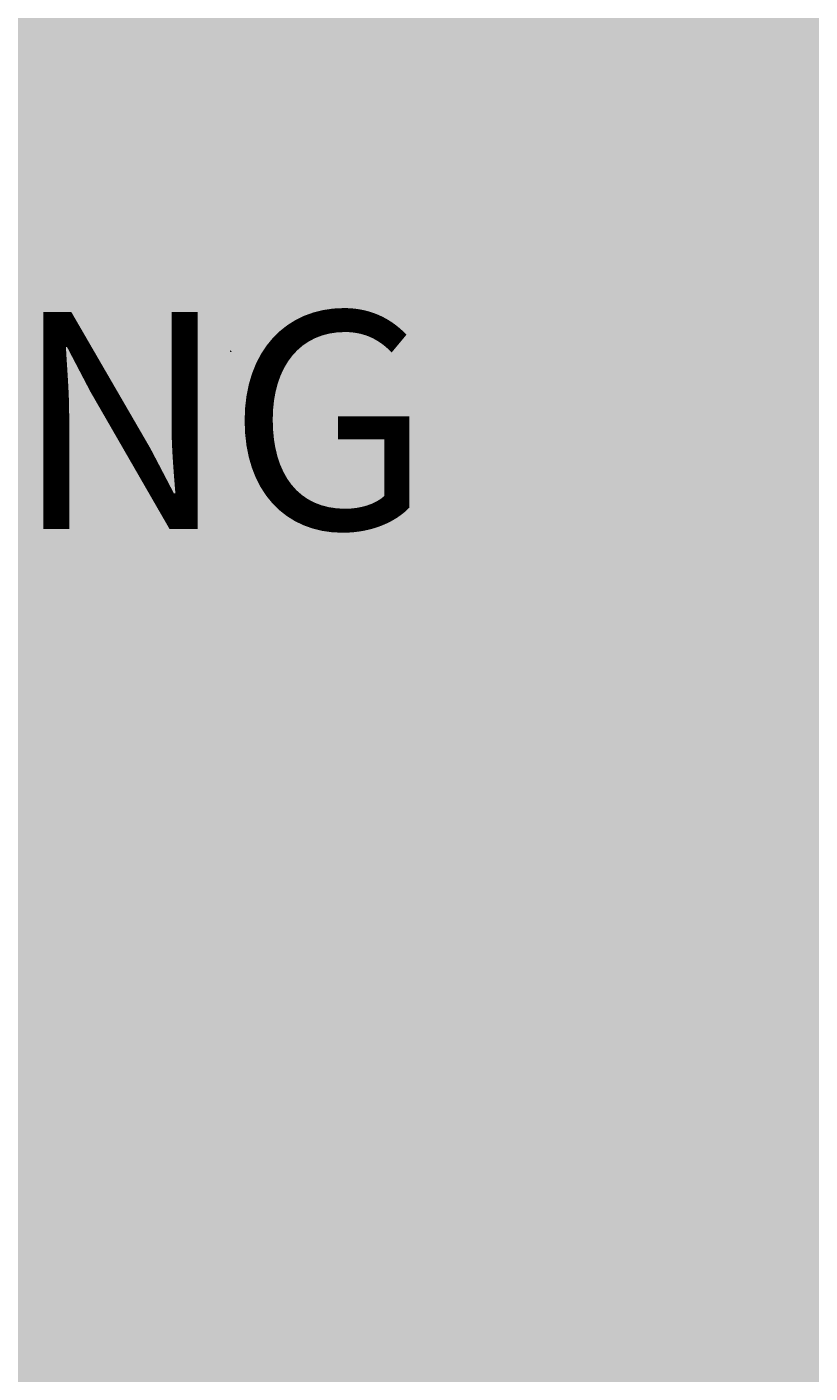
# Model space of a CAD drawing. Units: millimetres. Extents: x -229 to 16545, y -10488 to 4272.
# Tile 14 of 29: x 10978 to 11804, y -4126 to -2708. Entities that reach past the tile are written whole.
import ezdxf

# ---------------------------------------------------------------- set-up
doc = ezdxf.new("R2010")
doc.units = ezdxf.units.MM
doc.layers.add('A-ANNO-DIMS', color=2, linetype='Continuous', lineweight=18)
doc.layers.add('A-AREA-IDEN', color=7, linetype='Continuous', lineweight=18)
doc.layers.add('A-FLOR-PATT', color=254, linetype='Continuous', lineweight=13, true_color=0xfeeab9)
doc.styles.get("Standard").update_dxf_attribs({"font": 'arial.ttf'})
doc.dimstyles.get("Standard").update_dxf_attribs({"dimtxt": 0.18, "dimasz": 0.18, "dimexe": 0.18, "dimexo": 0.0625, "dimgap": 0.09, "dimtad": 0, "dimtih": 1, "dimtoh": 1, "dimdec": 4, "dimzin": 0, "dimdsep": 46, "dimtxsty": 'Standard', "dimcen": 0.09, "dimadec": 0, "dimazin": 0, "dimtfac": 1, "dimtdec": 4, "dimtofl": 0, "dimtmove": 0, "dimatfit": 3, "dimfxl": 1, "dimtolj": 1, "dimtzin": 0, "dimarcsym": 0})

# ---------------------------------------------------------------- blocks, each defined once
blk = doc.blocks.new('*D101')
at = {"layer": 'A-ANNO-DIMS', "color": 0, "lineweight": -2, "transparency": 16777216}
for p, q in [((10907.8, -3049.7), (10908, -3049.7)), ((10907.9, -3049.8), (10907.9, -3049.6)), ((15176.9, -3049.7), (13576.2, -3049.7))]:
    blk.add_line(p, q, dxfattribs=at)
at = {"layer": 'A-ANNO-DIMS', "color": 0, "transparency": 16777216}
blk.add_solid([(13576.2, -3049.7), (13576.2, -3049.7), (13576, -3049.7)], dxfattribs=at)
at = {"layer": 'Defpoints', "color": 0, "transparency": 16777216}
for p in [(10907.9, -3049.7), (13576, -3049.7)]:
    blk.add_point(p, dxfattribs=at)
at = {"layer": 'A-ANNO-DIMS', "color": 0, "transparency": 16777216, "insert": (15177.3, -3049.7), "char_height": 0.18, "attachment_point": 5}
blk.add_mtext('\\A1;R2668', dxfattribs=at)
blk = doc.blocks.new('*D102')
at = {"layer": 'A-ANNO-DIMS', "color": 0, "lineweight": -2, "transparency": 16777216}
for p, q in [((11192.8, -3049.7), (11193, -3049.7)), ((11192.9, -3049.8), (11192.9, -3049.6)), ((15217.2, -3049.7), (13708.3, -3049.7))]:
    blk.add_line(p, q, dxfattribs=at)
at = {"layer": 'A-ANNO-DIMS', "color": 0, "transparency": 16777216}
blk.add_solid([(13708.3, -3049.7), (13708.3, -3049.7), (13708.1, -3049.7)], dxfattribs=at)
at = {"layer": 'Defpoints', "color": 0, "transparency": 16777216}
for p in [(11192.9, -3049.7), (13708.1, -3049.7)]:
    blk.add_point(p, dxfattribs=at)
at = {"layer": 'A-ANNO-DIMS', "color": 0, "transparency": 16777216, "insert": (15217.6, -3049.7), "char_height": 0.18, "attachment_point": 5}
blk.add_mtext('\\A1;R2515', dxfattribs=at)

msp = doc.modelspace()

# ---------------------------------------------------------------- hatches: boundary and pattern name
at = {"layer": 'A-FLOR-PATT', "transparency": 33554592}
h = msp.add_hatch(color=256, dxfattribs=at)
h.dxf.hatch_style = 1
h.paths.add_polyline_path([(7975.933, -5325.772), (7943.121, -5325.772), (7943.121, -4576.49, 0.40145271), (7225.933, -5325.772, 0.40145271), (6508.746, -4576.49), (6508.746, -5325.772), (6475.933, -5325.772), (6475.933, -5438.272), (5975.933, -5438.272), (5975.933, -7267.724), (5975.933, -7438.272), (6478.619, -7438.272), (6463.448, -7355.919), (6464.88, -7356.837), (6463.849, -7358.097), (6478.619, -7438.272), (6610.327, -7438.272), (6632.656, -7409.564), (6632.525, -7406.967), (6634.208, -7407.569), (6619.273, -7426.77), (6654.466, -7438.272), (7610.517, -7438.272), (7607.41, -7421.409), (7608.842, -7422.327), (7607.812, -7423.587), (7610.517, -7438.272), (7975.933, -7438.272)])
h.paths.add_polyline_path([(13785.933, -1208.272), (9555.933, -1208.272), (9555.933, -961.785), (9705.933, -961.785), (9705.933, -918.035), (10704.976, -918.035, 0.40145271), (9705.933, 38.215), (9555.933, 38.215), (9555.933, 2021.728), (5975.933, 2021.728), (5975.933, 755.492), (5745.933, 755.492), (5745.933, 1427.266), (2918.813, 1427.266), (2918.813, -492.942), (5013.319, -492.942), (5013.319, -978.272), (5745.933, -978.272), (5745.933, -397.513), (5975.933, -397.513), (5975.933, -1208.272), (4560.933, -1208.272), (4560.933, -1265.772), (4448.433, -1265.772), (4448.433, -1298.585), (4445.933, -1298.585), (3699.151, -1298.585, 0.40145271), (4448.433, -2015.772), (4560.933, -2015.772), (4560.933, -2384.177), (5745.933, -2384.177), (5799.402, -2384.177), (5799.402, -4518.272), (5975.933, -4518.272), (5975.933, -5208.272), (6475.933, -5208.272), (6475.933, -4575.772), (6508.746, -4575.772), (6508.746, -4576.49, -0.35647263), (7216.672, -5208.272), (7235.194, -5208.272, -0.35647263), (7943.121, -4576.49), (7943.121, -4575.772), (7975.933, -4575.772), (7975.933, -5208.272), (11176.247, -5208.272), (11159.44, -5191.465), (10520.768, -5191.465), (10520.768, -4888.936), (10571.19, -4888.936), (10571.19, -4872.129), (10772.876, -4872.129), (10772.876, -4888.936), (10789.683, -4888.936), (10789.683, -4872.129), (10991.368, -4872.129), (10991.368, -4888.936), (11041.79, -4888.936), (11041.79, -4872.129), (11058.597, -4872.129, -0.09090909), (11428.354, -4872.129), (11445.162, -4872.129), (11445.162, -4888.936), (11529.197, -4888.936), (11529.197, -5191.465), (11327.512, -5191.465), (11310.704, -5208.272), (13785.933, -5208.272)])
h.paths.add_polyline_path([(11047.216, -1630.944, -1), (11402.816, -1630.944, -1)], flags=16)
h.paths.add_polyline_path([(11148.816, -1630.944), (11225.016, -1554.744), (11301.216, -1630.944), (11225.016, -1707.144)], flags=0)
h.paths.add_polyline_path([(11199.616, -1630.944, -1), (11250.416, -1630.944, -1)], flags=0)
h.paths.add_polyline_path([(11588.751, -2096.259), (11588.751, -1543.254, -0.26666697), (12864.918, -1543.254), (12864.918, -2096.259), (12737.302, -2096.259), (12737.302, -2063.121), (11716.368, -2063.121), (11716.368, -2096.259)], flags=16)
h.paths.add_polyline_path([(12012.696, -2489.42), (12600.997, -2489.42), (12600.997, -3666.022), (12012.696, -3666.022)], flags=16)
h.paths.add_polyline_path([(12176.41, -3599.403), (12174.938, -3609.076), (12173.789, -3618.819), (12173.09, -3628.559), (12172.973, -3638.221), (12173.89, -3652.852), (12175.008, -3657.025), (12172.909, -3643.473), (12173.142, -3624.297), (12175.386, -3605.273)], flags=0)
h.paths.add_polyline_path([(8026.289, -286.944), (7737.703, -287.19), (7734.87, -269.156), (8029.092, -268.905)], flags=16)
h.paths.add_polyline_path([(7733.453, -260.139), (7710.784, -115.865), (7557.191, -115.996), (7556.999, 109.744), (7412.687, 132.166), (7412.433, 429.206), (7556.707, 451.876), (7556.568, 614.769), (7412.256, 637.19), (7412.003, 934.231), (7556.276, 956.9), (7556.084, 1182.639), (7709.677, 1182.77), (7732.099, 1327.082), (8029.14, 1327.335), (8051.808, 1183.062), (8205.401, 1183.192), (8205.594, 957.454), (8349.906, 935.031), (8350.159, 637.99), (8205.885, 615.322), (8206.024, 452.43), (8350.336, 430.006), (8350.59, 132.965), (8206.316, 110.298), (8206.509, -115.442), (8052.916, -115.573), (8030.493, -259.885)], flags=16)
h.paths.add_polyline_path([(12261.416, -3475.554), (12262.632, -3486.776), (12264.032, -3497.007), (12265.554, -3506.365), (12267.136, -3514.968), (12268.719, -3522.935), (12271.304, -3535.59), (12273.606, -3548.078), (12275.271, -3561.064), (12275.93, -3574.938), (12275.325, -3590.3), (12273.425, -3607.964), (12270.795, -3625.658), (12268.066, -3641.063), (12266.318, -3649.679), (12265.456, -3653.626), (12263.984, -3659.846), (12264.032, -3659.566), (12264.342, -3658.241), (12264.807, -3656.37), (12265.456, -3653.626), (12266.318, -3649.679), (12267.409, -3644.302), (12268.668, -3637.664), (12270.019, -3630.037), (12271.384, -3621.695), (12272.69, -3612.908), (12273.857, -3603.948), (12274.81, -3595.088), (12275.47, -3586.601), (12275.782, -3578.689), (12275.757, -3571.292), (12275.423, -3564.275), (12274.816, -3557.512), (12273.964, -3550.872), (12272.896, -3544.224), (12271.645, -3537.439), (12270.24, -3530.385), (12267.543, -3517.181), (12264.612, -3501.247), (12261.849, -3481.059)], flags=0)
h.paths.add_polyline_path([(12332.136, -3408.03), (12333.483, -3416.79), (12335.077, -3424.54), (12336.915, -3431.355), (12338.991, -3437.32), (12341.266, -3442.55), (12343.694, -3447.166), (12346.229, -3451.292), (12348.826, -3455.051), (12351.438, -3458.563), (12357.476, -3466.491), (12363.61, -3476.575), (12368.309, -3489.762), (12369.929, -3503.427), (12369.842, -3516.511), (12368.43, -3530.867), (12365.816, -3545.835), (12362.382, -3559.786), (12360.968, -3564.487), (12363.063, -3557.021), (12364.898, -3549.566), (12366.473, -3542.077), (12367.773, -3534.631), (12368.781, -3527.301), (12369.483, -3520.162), (12369.863, -3513.291), (12369.906, -3506.759), (12369.599, -3500.643), (12368.93, -3494.999), (12367.924, -3489.796), (12366.61, -3484.994), (12365.024, -3480.542), (12363.19, -3476.399), (12361.141, -3472.516), (12358.909, -3468.847), (12356.525, -3465.347), (12354.02, -3461.954), (12351.438, -3458.563), (12345.462, -3450.529), (12339.923, -3439.996), (12335.85, -3428.296), (12332.68, -3412.888)], flags=0)
h.paths.add_polyline_path([(12385.287, -3334.612), (12384.977, -3342.409), (12385.02, -3349.196), (12385.4, -3355.066), (12386.104, -3360.105), (12387.112, -3364.41), (12388.412, -3368.071), (12389.987, -3371.181), (12391.823, -3373.832), (12393.919, -3376.097), (12396.337, -3377.978), (12399.153, -3379.462), (12402.445, -3380.531), (12406.289, -3381.172), (12410.758, -3381.371), (12415.935, -3381.106), (12421.893, -3380.368), (12428.658, -3379.159), (12436.069, -3377.55), (12443.907, -3375.635), (12451.961, -3373.505), (12460.015, -3371.254), (12467.853, -3368.971), (12475.263, -3366.749), (12482.029, -3364.68), (12491.877, -3361.657), (12497.701, -3360.107), (12501.639, -3359.288), (12510.135, -3358.326), (12519.662, -3365.412), (12524.243, -3378.911), (12523.764, -3390.7), (12520.746, -3401.577), (12514.248, -3415.634), (12511.518, -3420.418), (12515.856, -3412.154), (12519.153, -3405.024), (12521.516, -3398.804), (12523.049, -3393.276), (12523.865, -3388.212), (12524.059, -3383.441), (12523.7, -3378.958), (12522.853, -3374.815), (12521.576, -3371.054), (12519.931, -3367.722), (12517.982, -3364.865), (12515.786, -3362.529), (12513.405, -3360.758), (12510.877, -3359.588), (12508.136, -3358.982), (12505.086, -3358.897), (12501.639, -3359.288), (12497.701, -3360.107), (12493.183, -3361.309), (12487.988, -3362.851), (12476.403, -3366.408), (12463.335, -3370.326), (12447.372, -3374.788), (12431.759, -3378.604), (12418.504, -3380.974), (12405.811, -3381.624), (12394.725, -3378.025), (12388.039, -3368.367), (12385.583, -3357.877), (12384.826, -3346.204), (12385.428, -3331.059), (12385.953, -3325.719)], flags=0)
h.paths.add_polyline_path([(7880.016, 1173.969), (7880.373, 1175.495), (7880.433, 1175.851), (7879.484, 1171.818)], flags=0)
h.paths.add_polyline_path([(7802.33, 874.962), (7800.771, 885.032), (7798.932, 893.941), (7796.811, 901.774), (7794.419, 908.63), (7791.798, 914.639), (7789.002, 919.945), (7786.083, 924.686), (7783.093, 929.005), (7780.087, 933.043), (7774.996, 939.717), (7768.406, 949.37), (7762.174, 963.427), (7759.342, 978.002), (7758.629, 991.888), (7759.492, 1007.928), (7761.801, 1025.496), (7765.392, 1044.035), (7766.625, 1049.048), (7764.522, 1039.543), (7762.719, 1030.232), (7761.232, 1021.168), (7760.08, 1012.405), (7759.28, 1003.994), (7758.849, 995.988), (7758.806, 988.44), (7759.167, 981.404), (7759.942, 974.914), (7761.104, 968.936), (7762.617, 963.414), (7764.448, 958.299), (7766.559, 953.535), (7768.918, 949.073), (7771.487, 944.856), (7774.232, 940.835), (7777.115, 936.938), (7782.377, 930.041), (7787.845, 922.139), (7793.348, 911.698), (7798.042, 898.247), (7801.702, 880.527)], flags=0)
h.paths.add_polyline_path([(12519.068, -3228.534), (12519.615, -3236.235), (12520.529, -3242.343), (12521.78, -3247.103), (12523.337, -3250.758), (12525.171, -3253.556), (12527.248, -3255.709), (12529.522, -3257.296), (12531.95, -3258.361), (12534.486, -3258.949), (12537.082, -3259.11), (12539.694, -3258.888), (12542.277, -3258.329), (12544.781, -3257.478), (12547.173, -3256.388), (12549.46, -3255.129), (12550.455, -3254.517), (12555.825, -3251.109), (12557.835, -3249.942), (12565.181, -3246.404), (12574.565, -3253.032), (12576.931, -3265.022), (12576.627, -3277.425), (12575.416, -3290.819), (12574.851, -3295.392), (12575.708, -3287.593), (12576.322, -3280.806), (12576.688, -3274.939), (12576.812, -3269.899), (12576.688, -3265.593), (12576.322, -3261.932), (12575.708, -3258.822), (12574.851, -3256.172), (12573.753, -3253.905), (12572.439, -3252.005), (12570.943, -3250.474), (12569.293, -3249.309), (12567.523, -3248.513), (12565.658, -3248.083), (12563.732, -3248.022), (12561.777, -3248.328), (12559.814, -3248.989), (12557.835, -3249.942), (12555.825, -3251.109), (12553.77, -3252.413), (12551.652, -3253.78), (12549.46, -3255.129), (12543.167, -3258.594), (12532.661, -3259.485), (12524.685, -3253.923), (12520.949, -3245.152), (12519.138, -3233.042)], flags=0)
h.paths.add_polyline_path([(7741.293, 790.501), (7741.641, 799.467), (7741.584, 807.269), (7741.141, 814.015), (7740.329, 819.809), (7739.165, 824.757), (7737.667, 828.966), (7735.853, 832.541), (7733.74, 835.586), (7731.348, 838.188), (7728.71, 840.348), (7725.861, 842.052), (7722.836, 843.28), (7719.671, 844.015), (7716.4, 844.237), (7713.06, 843.932), (7709.684, 843.081), (7706.304, 841.686), (7702.923, 839.834), (7699.543, 837.629), (7696.164, 835.178), (7692.784, 832.585), (7684.718, 826.315), (7675.609, 820.63), (7664.001, 817.274), (7654.105, 821.884), (7647.171, 832.02), (7644.191, 846.522), (7646.321, 860.288), (7647.49, 864.223), (7645.946, 857.865), (7645.046, 852.044), (7644.827, 846.557), (7645.243, 841.404), (7646.221, 836.642), (7647.693, 832.318), (7649.587, 828.489), (7651.832, 825.206), (7654.359, 822.523), (7657.097, 820.49), (7659.984, 819.145), (7662.993, 818.452), (7666.108, 818.357), (7669.311, 818.809), (7672.583, 819.755), (7675.908, 821.139), (7679.268, 822.913), (7682.645, 825.021), (7686.025, 827.401), (7689.404, 829.958), (7692.784, 832.585), (7700.505, 838.509), (7709.871, 843.64), (7721.436, 844.698), (7733.277, 837.617), (7739.571, 825.214), (7741.557, 811.049), (7741.669, 795.575)], flags=0)
h.paths.add_polyline_path([(8377.641, 137.216), (8359.607, 134.382), (8359.356, 428.605), (8377.395, 425.802)], flags=16)
h.paths.add_polyline_path([(7650.715, 668.465), (7650.08, 677.319), (7649.023, 684.34), (7647.579, 689.811), (7645.785, 694.012), (7643.675, 697.228), (7641.286, 699.7), (7638.669, 701.521), (7635.876, 702.744), (7632.96, 703.419), (7629.974, 703.601), (7626.971, 703.344), (7624.004, 702.697), (7621.125, 701.717), (7618.375, 700.462), (7615.749, 699.013), (7614.561, 698.279), (7608.435, 694.382), (7606.125, 693.04), (7598.981, 689.594), (7589.669, 693.773), (7585.26, 702.856), (7584.221, 713.11), (7584.49, 724.584), (7585.863, 739.937), (7586.518, 745.277), (7585.539, 736.31), (7584.841, 728.507), (7584.424, 721.761), (7584.288, 715.966), (7584.433, 711.016), (7584.86, 706.807), (7585.567, 703.231), (7586.556, 700.186), (7587.821, 697.58), (7589.332, 695.397), (7591.053, 693.637), (7592.951, 692.3), (7594.989, 691.385), (7597.132, 690.895), (7599.346, 690.826), (7601.594, 691.18), (7603.851, 691.943), (7606.125, 693.04), (7608.435, 694.382), (7610.797, 695.885), (7613.229, 697.458), (7620.475, 701.929), (7632.001, 704.44), (7643.476, 699.417), (7648.536, 687.571), (7650.63, 673.661)], flags=0)
h.paths.add_polyline_path([(7385.628, 136.37), (7385.382, 424.956), (7403.416, 427.789), (7403.667, 133.567)], flags=16)
h.paths.add_polyline_path([(12993.884, -2257.186), (12959.588, -2257.186), (12959.588, -2125.099), (13531.966, -2125.099, -0.19047621), (13531.966, -3974.321), (12959.588, -3974.321), (12959.588, -3842.233), (12993.884, -3842.233)], flags=16)
h.paths.add_polyline_path([(13413.486, -3313.884), (13413.486, -2785.535), (13562.885, -2785.535, -0.04962821), (13562.885, -3313.884)], flags=0)
h.paths.add_polyline_path([(8377.21, 642.241), (8359.176, 639.407), (8358.925, 933.629), (8376.964, 930.826)], flags=16)
h.paths.add_polyline_path([(13086.058, -1864.83), (13086.058, -1449.84), (13501.048, -1449.84), (13501.048, -1864.83)], flags=16)
h.paths.add_polyline_path([(13305.814, -1862.197), (13302.103, -1859.624), (13298.088, -1857.068), (13293.799, -1854.536), (13289.262, -1852.031), (13284.504, -1849.559), (13279.554, -1847.125), (13274.439, -1844.735), (13269.17, -1842.389), (13263.701, -1840.081), (13257.97, -1837.797), (13251.914, -1835.525), (13245.472, -1833.252), (13238.582, -1830.968), (13231.18, -1828.66), (13223.206, -1826.315), (13209.182, -1822.458), (13204.584, -1821.48), (13217.962, -1824.773), (13235.072, -1829.804), (13248.777, -1834.349), (13260.829, -1838.869), (13274.479, -1844.63), (13289.675, -1852.101), (13302.553, -1859.704)], flags=0)
h.paths.add_polyline_path([(13428.104, -1820.994), (13419.007, -1818.141), (13409.95, -1815.4), (13400.766, -1812.747), (13391.271, -1810.151), (13376.087, -1806.251), (13370.618, -1805.019), (13386.304, -1808.794), (13405.087, -1813.928), (13423.014, -1819.354)], flags=0)
h.paths.add_polyline_path([(7385.197, 641.395), (7384.951, 929.98), (7402.986, 932.814), (7403.236, 638.592)], flags=16)
h.paths.add_polyline_path([(13262.537, -1725.526), (13253.246, -1724.74), (13244.516, -1724.117), (13235.94, -1723.625), (13223.267, -1723.062), (13217.598, -1722.912), (13231.966, -1723.397), (13248.733, -1724.359), (13266.899, -1725.895), (13272.802, -1726.502)], flags=0)
h.paths.add_polyline_path([(13191.893, -1641.137), (13208.675, -1640.506), (13214.057, -1640.258), (13197.763, -1640.936)], flags=0)
h.paths.add_polyline_path([(13097.524, -1608.457), (13114.284, -1609.031), (13120.126, -1609.105), (13103.045, -1608.71)], flags=0)
h.paths.add_polyline_path([(13465.328, -1521.577), (13473.906, -1517.015), (13481.761, -1511.636), (13492.562, -1502.076), (13495.327, -1497.933), (13485.818, -1508.858), (13470.208, -1519.547)], flags=0)
h.paths.add_polyline_path([(13175.015, -1500.891), (13184.046, -1501.807), (13192.721, -1502.52), (13201.114, -1503.034), (13209.273, -1503.351), (13217.244, -1503.476), (13225.078, -1503.41), (13232.821, -1503.16), (13240.524, -1502.728), (13248.233, -1502.117), (13255.993, -1501.322), (13263.825, -1500.293), (13271.746, -1498.974), (13279.775, -1497.305), (13287.928, -1495.229), (13296.222, -1492.688), (13304.675, -1489.622), (13313.304, -1485.975), (13322.089, -1481.727), (13330.859, -1477.028), (13339.408, -1472.063), (13347.526, -1467.02), (13355.006, -1462.087), (13364.86, -1455.202), (13367.224, -1453.299), (13358.544, -1459.754), (13343.348, -1469.775), (13326.143, -1479.767), (13309.023, -1488.045), (13292.249, -1494.129), (13276.009, -1498.264), (13260.299, -1500.88), (13244.401, -1502.51), (13228.945, -1503.378), (13213.316, -1503.508), (13197.047, -1502.876), (13180.088, -1501.481)], flags=0)
h.paths.add_polyline_path([(7733.501, 1336.101), (7736.303, 1354.14), (8024.889, 1354.386), (8027.723, 1336.352)], flags=16)

# ---------------------------------------------------------------- texts
at = {"layer": 'A-AREA-IDEN'}
msp.add_text('LIVING', height=228.5841, dxfattribs=at).set_placement((10432.603, -3236.78))

# ---------------------------------------------------------------- dimensions: what is measured, and where the dimension line sits
at = {"layer": 'A-ANNO-DIMS'}
for center, mpoint, picture, middle in [((10907.903, -3049.71), (13575.995, -3049.709), '*D101', (15176.85, -3049.708)), ((11192.921, -3049.71), (13708.082, -3049.71), '*D102', (15217.179, -3049.71))]:
    dim = msp.add_radius_dim(center=center, mpoint=mpoint, dimstyle='Standard', override={"dimdec": 0, "dimlfac": 1, "dimrnd": 0, "dimzin": 0, "dimdsep": 46, "dimlunit": 2}, dxfattribs=at)
    dim.commit()
    dim.dimension.update_dxf_attribs({"geometry": picture, "text_midpoint": middle, "dimtype": 164})

doc.saveas('drawing.dxf')
